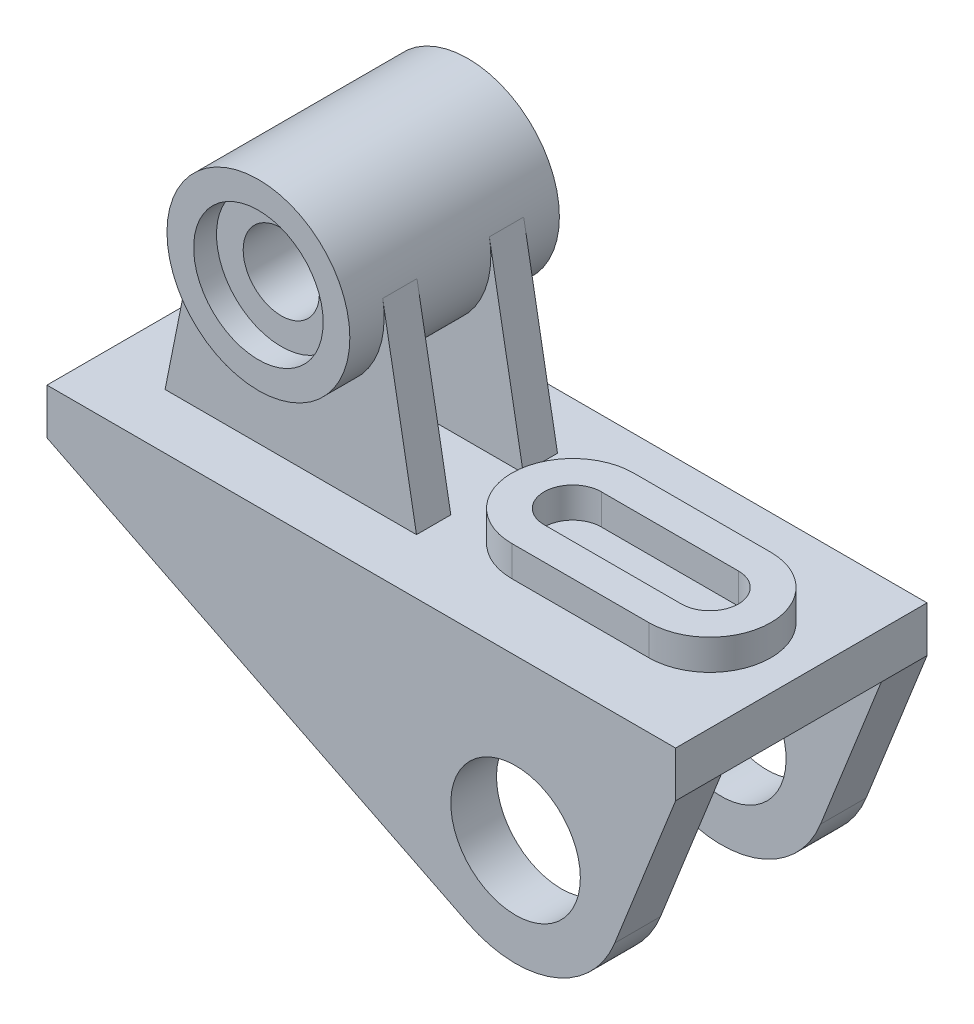
ISO-10303-21;
HEADER;
FILE_DESCRIPTION(('STEP AP214'),'2;1');
FILE_NAME('part.step','',(''),(''),'','','');
FILE_SCHEMA(('AUTOMOTIVE_DESIGN { 1 0 10303 214 1 1 1 1 }'));
ENDSEC;
DATA;
#1=APPLICATION_CONTEXT('core data for automotive mechanical design processes');
#2=APPLICATION_PROTOCOL_DEFINITION('international standard','automotive_design',2000,#1);
#3=PRODUCT_CONTEXT('',#1,'mechanical');
#4=PRODUCT('Part','Part','',(#3));
#5=PRODUCT_RELATED_PRODUCT_CATEGORY('part','',(#4));
#6=PRODUCT_DEFINITION_FORMATION('','',#4);
#7=PRODUCT_DEFINITION_CONTEXT('part definition',#1,'design');
#8=PRODUCT_DEFINITION('design','',#6,#7);
#9=PRODUCT_DEFINITION_SHAPE('','',#8);
#10=(LENGTH_UNIT() NAMED_UNIT(*) SI_UNIT(.MILLI.,.METRE.));
#11=(NAMED_UNIT(*) PLANE_ANGLE_UNIT() SI_UNIT($,.RADIAN.));
#12=(NAMED_UNIT(*) SI_UNIT($,.STERADIAN.) SOLID_ANGLE_UNIT());
#13=UNCERTAINTY_MEASURE_WITH_UNIT(LENGTH_MEASURE(1.E-05),#10,'distance_accuracy_value','');
#14=(GEOMETRIC_REPRESENTATION_CONTEXT(3) GLOBAL_UNCERTAINTY_ASSIGNED_CONTEXT((#13)) GLOBAL_UNIT_ASSIGNED_CONTEXT((#10,
#11,#12)) REPRESENTATION_CONTEXT('',''));
#15=CARTESIAN_POINT('',(0.,0.,0.));
#16=DIRECTION('',(0.,0.,1.));
#17=DIRECTION('',(1.,0.,0.));
#18=AXIS2_PLACEMENT_3D('',#15,#16,#17);
#19=CARTESIAN_POINT('',(50.,45.,27.5));
#20=DIRECTION('',(0.,0.,-1.));
#21=DIRECTION('',(-1.,0.,0.));
#22=AXIS2_PLACEMENT_3D('',#19,#20,#21);
#23=CYLINDRICAL_SURFACE('',#22,9.99999999999999);
#24=CARTESIAN_POINT('',(50.,45.,21.5));
#25=DIRECTION('',(0.,0.,1.));
#26=DIRECTION('',(1.,0.,0.));
#27=AXIS2_PLACEMENT_3D('',#24,#25,#26);
#28=CIRCLE('',#27,9.99999999999999);
#29=CARTESIAN_POINT('',(60.,45.,21.5));
#30=VERTEX_POINT('',#29);
#31=EDGE_CURVE('E248',#30,#30,#28,.T.);
#32=ORIENTED_EDGE('',*,*,#31,.T.);
#33=EDGE_LOOP('',(#32));
#34=FACE_BOUND('',#33,.T.);
#35=CARTESIAN_POINT('',(50.,45.,-21.5));
#36=DIRECTION('',(0.,0.,-1.));
#37=DIRECTION('',(-1.,0.,0.));
#38=AXIS2_PLACEMENT_3D('',#35,#36,#37);
#39=CIRCLE('',#38,9.99999999999999);
#40=CARTESIAN_POINT('',(40.,45.,-21.5));
#41=VERTEX_POINT('',#40);
#42=EDGE_CURVE('E43',#41,#41,#39,.T.);
#43=ORIENTED_EDGE('',*,*,#42,.T.);
#44=EDGE_LOOP('',(#43));
#45=FACE_BOUND('',#44,.T.);
#46=ADVANCED_FACE('F39',(#34,#45),#23,.F.);
#47=CARTESIAN_POINT('',(0.,0.,33.));
#48=DIRECTION('',(0.,-1.,0.));
#49=DIRECTION('',(0.,0.,-1.));
#50=AXIS2_PLACEMENT_3D('',#47,#48,#49);
#51=PLANE('',#50);
#52=DIRECTION('',(1.,0.,0.));
#53=VECTOR('',#52,1.);
#54=CARTESIAN_POINT('',(16.5,0.,9.5));
#55=LINE('',#54,#53);
#56=CARTESIAN_POINT('',(16.5,0.,9.5));
#57=VERTEX_POINT('',#56);
#58=CARTESIAN_POINT('',(82.5,0.,9.5));
#59=VERTEX_POINT('',#58);
#60=EDGE_CURVE('E268',#57,#59,#55,.T.);
#61=ORIENTED_EDGE('',*,*,#60,.T.);
#62=DIRECTION('',(0.,0.,1.));
#63=VECTOR('',#62,1.);
#64=CARTESIAN_POINT('',(82.5,0.,9.5));
#65=LINE('',#64,#63);
#66=CARTESIAN_POINT('',(82.5,0.,18.5));
#67=VERTEX_POINT('',#66);
#68=EDGE_CURVE('E289',#59,#67,#65,.T.);
#69=ORIENTED_EDGE('',*,*,#68,.T.);
#70=DIRECTION('',(1.,0.,0.));
#71=VECTOR('',#70,1.);
#72=CARTESIAN_POINT('',(16.5,0.,18.5));
#73=LINE('',#72,#71);
#74=CARTESIAN_POINT('',(16.5,0.,18.5));
#75=VERTEX_POINT('',#74);
#76=EDGE_CURVE('E276',#75,#67,#73,.T.);
#77=ORIENTED_EDGE('',*,*,#76,.F.);
#78=DIRECTION('',(0.,0.,1.));
#79=VECTOR('',#78,1.);
#80=CARTESIAN_POINT('',(16.5,0.,9.5));
#81=LINE('',#80,#79);
#82=EDGE_CURVE('E286',#57,#75,#81,.T.);
#83=ORIENTED_EDGE('',*,*,#82,.F.);
#84=EDGE_LOOP('',(#61,#69,#77,#83));
#85=FACE_BOUND('',#84,.T.);
#86=DIRECTION('',(-1.,0.,0.));
#87=VECTOR('',#86,1.);
#88=CARTESIAN_POINT('',(0.,0.,-33.));
#89=LINE('',#88,#87);
#90=CARTESIAN_POINT('',(165.,0.,-33.));
#91=VERTEX_POINT('',#90);
#92=CARTESIAN_POINT('',(0.,0.,-33.));
#93=VERTEX_POINT('',#92);
#94=EDGE_CURVE('E398',#91,#93,#89,.T.);
#95=ORIENTED_EDGE('',*,*,#94,.T.);
#96=DIRECTION('',(0.,0.,-1.));
#97=VECTOR('',#96,1.);
#98=CARTESIAN_POINT('',(0.,0.,33.));
#99=LINE('',#98,#97);
#100=CARTESIAN_POINT('',(0.,0.,33.));
#101=VERTEX_POINT('',#100);
#102=EDGE_CURVE('E408',#101,#93,#99,.T.);
#103=ORIENTED_EDGE('',*,*,#102,.F.);
#104=DIRECTION('',(-1.,0.,0.));
#105=VECTOR('',#104,1.);
#106=CARTESIAN_POINT('',(0.,0.,33.));
#107=LINE('',#106,#105);
#108=CARTESIAN_POINT('',(165.,0.,33.));
#109=VERTEX_POINT('',#108);
#110=EDGE_CURVE('E404',#109,#101,#107,.T.);
#111=ORIENTED_EDGE('',*,*,#110,.F.);
#112=DIRECTION('',(0.,0.,-1.));
#113=VECTOR('',#112,1.);
#114=CARTESIAN_POINT('',(165.,0.,33.));
#115=LINE('',#114,#113);
#116=EDGE_CURVE('E421',#109,#91,#115,.T.);
#117=ORIENTED_EDGE('',*,*,#116,.T.);
#118=EDGE_LOOP('',(#95,#103,#111,#117));
#119=FACE_BOUND('',#118,.T.);
#120=CARTESIAN_POINT('',(105.,0.,0.));
#121=DIRECTION('',(0.,1.,0.));
#122=DIRECTION('',(0.,0.,1.));
#123=AXIS2_PLACEMENT_3D('',#120,#121,#122);
#124=CIRCLE('',#123,16.);
#125=CARTESIAN_POINT('',(105.,0.,-16.));
#126=VERTEX_POINT('',#125);
#127=CARTESIAN_POINT('',(105.,0.,16.));
#128=VERTEX_POINT('',#127);
#129=EDGE_CURVE('E323',#126,#128,#124,.T.);
#130=ORIENTED_EDGE('',*,*,#129,.F.);
#131=DIRECTION('',(-1.,0.,0.));
#132=VECTOR('',#131,1.);
#133=CARTESIAN_POINT('',(105.,0.,-16.));
#134=LINE('',#133,#132);
#135=CARTESIAN_POINT('',(141.,0.,-16.));
#136=VERTEX_POINT('',#135);
#137=EDGE_CURVE('E327',#136,#126,#134,.T.);
#138=ORIENTED_EDGE('',*,*,#137,.F.);
#139=CARTESIAN_POINT('',(141.,0.,0.));
#140=DIRECTION('',(0.,1.,0.));
#141=DIRECTION('',(0.,0.,1.));
#142=AXIS2_PLACEMENT_3D('',#139,#140,#141);
#143=CIRCLE('',#142,16.);
#144=CARTESIAN_POINT('',(141.,0.,16.));
#145=VERTEX_POINT('',#144);
#146=EDGE_CURVE('E337',#145,#136,#143,.T.);
#147=ORIENTED_EDGE('',*,*,#146,.F.);
#148=DIRECTION('',(1.,0.,0.));
#149=VECTOR('',#148,1.);
#150=CARTESIAN_POINT('',(105.,0.,16.));
#151=LINE('',#150,#149);
#152=EDGE_CURVE('E340',#128,#145,#151,.T.);
#153=ORIENTED_EDGE('',*,*,#152,.F.);
#154=EDGE_LOOP('',(#130,#138,#147,#153));
#155=FACE_BOUND('',#154,.T.);
#156=DIRECTION('',(1.,0.,0.));
#157=VECTOR('',#156,1.);
#158=CARTESIAN_POINT('',(16.5,0.,-9.5));
#159=LINE('',#158,#157);
#160=CARTESIAN_POINT('',(16.5,0.,-9.5));
#161=VERTEX_POINT('',#160);
#162=CARTESIAN_POINT('',(82.5,0.,-9.5));
#163=VERTEX_POINT('',#162);
#164=EDGE_CURVE('E222',#161,#163,#159,.T.);
#165=ORIENTED_EDGE('',*,*,#164,.F.);
#166=DIRECTION('',(0.,0.,-1.));
#167=VECTOR('',#166,1.);
#168=CARTESIAN_POINT('',(16.5,0.,-9.5));
#169=LINE('',#168,#167);
#170=CARTESIAN_POINT('',(16.5,0.,-18.5));
#171=VERTEX_POINT('',#170);
#172=EDGE_CURVE('E252',#161,#171,#169,.T.);
#173=ORIENTED_EDGE('',*,*,#172,.T.);
#174=DIRECTION('',(1.,0.,0.));
#175=VECTOR('',#174,1.);
#176=CARTESIAN_POINT('',(16.5,0.,-18.5));
#177=LINE('',#176,#175);
#178=CARTESIAN_POINT('',(82.5,0.,-18.5));
#179=VERTEX_POINT('',#178);
#180=EDGE_CURVE('E237',#171,#179,#177,.T.);
#181=ORIENTED_EDGE('',*,*,#180,.T.);
#182=DIRECTION('',(0.,0.,-1.));
#183=VECTOR('',#182,1.);
#184=CARTESIAN_POINT('',(82.5,0.,-9.5));
#185=LINE('',#184,#183);
#186=EDGE_CURVE('E227',#163,#179,#185,.T.);
#187=ORIENTED_EDGE('',*,*,#186,.F.);
#188=EDGE_LOOP('',(#165,#173,#181,#187));
#189=FACE_BOUND('',#188,.T.);
#190=ADVANCED_FACE('F472',(#85,#119,#155,#189),#51,.F.);
#191=CARTESIAN_POINT('',(50.,45.,27.5));
#192=DIRECTION('',(0.,0.,-1.));
#193=DIRECTION('',(-1.,0.,0.));
#194=AXIS2_PLACEMENT_3D('',#191,#192,#193);
#195=CYLINDRICAL_SURFACE('',#194,24.);
#196=DIRECTION('',(0.,0.,1.));
#197=VECTOR('',#196,1.);
#198=CARTESIAN_POINT('',(73.6192033310231,49.25831351685,9.5));
#199=LINE('',#198,#197);
#200=CARTESIAN_POINT('',(73.6192033310231,49.25831351685,9.50000000000001));
#201=VERTEX_POINT('',#200);
#202=CARTESIAN_POINT('',(73.6192033310231,49.25831351685,18.5));
#203=VERTEX_POINT('',#202);
#204=EDGE_CURVE('E281',#201,#203,#199,.T.);
#205=ORIENTED_EDGE('',*,*,#204,.F.);
#206=CARTESIAN_POINT('',(50.,45.,9.5));
#207=DIRECTION('',(0.,0.,-1.));
#208=DIRECTION('',(1.,0.,0.));
#209=AXIS2_PLACEMENT_3D('',#206,#207,#208);
#210=CIRCLE('',#209,24.);
#211=CARTESIAN_POINT('',(26.4683154892939,49.7180318024145,9.50000000000001));
#212=VERTEX_POINT('',#211);
#213=EDGE_CURVE('E265',#201,#212,#210,.T.);
#214=ORIENTED_EDGE('',*,*,#213,.T.);
#215=DIRECTION('',(0.,0.,1.));
#216=VECTOR('',#215,1.);
#217=CARTESIAN_POINT('',(26.4683154892939,49.7180318024145,9.5));
#218=LINE('',#217,#216);
#219=CARTESIAN_POINT('',(26.4683154892939,49.7180318024145,18.5));
#220=VERTEX_POINT('',#219);
#221=EDGE_CURVE('E273',#212,#220,#218,.T.);
#222=ORIENTED_EDGE('',*,*,#221,.T.);
#223=CARTESIAN_POINT('',(50.,45.,18.5));
#224=DIRECTION('',(0.,0.,-1.));
#225=DIRECTION('',(1.,0.,0.));
#226=AXIS2_PLACEMENT_3D('',#223,#224,#225);
#227=CIRCLE('',#226,24.);
#228=EDGE_CURVE('E259',#203,#220,#227,.T.);
#229=ORIENTED_EDGE('',*,*,#228,.F.);
#230=EDGE_LOOP('',(#205,#214,#222,#229));
#231=FACE_BOUND('',#230,.T.);
#232=CARTESIAN_POINT('',(50.,45.,-27.5));
#233=DIRECTION('',(0.,0.,1.));
#234=DIRECTION('',(1.,0.,0.));
#235=AXIS2_PLACEMENT_3D('',#232,#233,#234);
#236=CIRCLE('',#235,24.);
#237=CARTESIAN_POINT('',(74.,45.,-27.5));
#238=VERTEX_POINT('',#237);
#239=EDGE_CURVE('E253',#238,#238,#236,.T.);
#240=ORIENTED_EDGE('',*,*,#239,.T.);
#241=EDGE_LOOP('',(#240));
#242=FACE_BOUND('',#241,.T.);
#243=CARTESIAN_POINT('',(50.,45.,27.5));
#244=DIRECTION('',(0.,0.,1.));
#245=DIRECTION('',(1.,0.,0.));
#246=AXIS2_PLACEMENT_3D('',#243,#244,#245);
#247=CIRCLE('',#246,24.);
#248=CARTESIAN_POINT('',(74.,45.,27.5));
#249=VERTEX_POINT('',#248);
#250=EDGE_CURVE('E258',#249,#249,#247,.T.);
#251=ORIENTED_EDGE('',*,*,#250,.F.);
#252=EDGE_LOOP('',(#251));
#253=FACE_BOUND('',#252,.T.);
#254=CARTESIAN_POINT('',(50.,45.,-9.5));
#255=DIRECTION('',(0.,0.,-1.));
#256=DIRECTION('',(1.,0.,0.));
#257=AXIS2_PLACEMENT_3D('',#254,#255,#256);
#258=CIRCLE('',#257,24.);
#259=CARTESIAN_POINT('',(73.6192033310231,49.25831351685,-9.5));
#260=VERTEX_POINT('',#259);
#261=CARTESIAN_POINT('',(26.4683154892939,49.7180318024145,-9.5));
#262=VERTEX_POINT('',#261);
#263=EDGE_CURVE('E218',#260,#262,#258,.T.);
#264=ORIENTED_EDGE('',*,*,#263,.F.);
#265=DIRECTION('',(0.,0.,-1.));
#266=VECTOR('',#265,1.);
#267=CARTESIAN_POINT('',(73.6192033310231,49.25831351685,-9.5));
#268=LINE('',#267,#266);
#269=CARTESIAN_POINT('',(73.6192033310231,49.25831351685,-18.5));
#270=VERTEX_POINT('',#269);
#271=EDGE_CURVE('E228',#260,#270,#268,.T.);
#272=ORIENTED_EDGE('',*,*,#271,.T.);
#273=CARTESIAN_POINT('',(50.,45.,-18.5));
#274=DIRECTION('',(0.,0.,-1.));
#275=DIRECTION('',(1.,0.,0.));
#276=AXIS2_PLACEMENT_3D('',#273,#274,#275);
#277=CIRCLE('',#276,24.);
#278=CARTESIAN_POINT('',(26.4683154892939,49.7180318024145,-18.5));
#279=VERTEX_POINT('',#278);
#280=EDGE_CURVE('E244',#270,#279,#277,.T.);
#281=ORIENTED_EDGE('',*,*,#280,.T.);
#282=DIRECTION('',(0.,0.,-1.));
#283=VECTOR('',#282,1.);
#284=CARTESIAN_POINT('',(26.4683154892939,49.7180318024145,-9.5));
#285=LINE('',#284,#283);
#286=EDGE_CURVE('E64',#262,#279,#285,.T.);
#287=ORIENTED_EDGE('',*,*,#286,.F.);
#288=EDGE_LOOP('',(#264,#272,#281,#287));
#289=FACE_BOUND('',#288,.T.);
#290=ADVANCED_FACE('F232',(#231,#242,#253,#289),#195,.T.);
#291=CARTESIAN_POINT('',(0.,-12.,33.));
#292=DIRECTION('',(0.445949175153248,0.895058284794983,0.));
#293=DIRECTION('',(-0.895058284794984,0.445949175153248,0.));
#294=AXIS2_PLACEMENT_3D('',#291,#292,#293);
#295=PLANE('',#294);
#296=DIRECTION('',(0.,0.,-1.));
#297=VECTOR('',#296,1.);
#298=CARTESIAN_POINT('',(0.,-12.,33.));
#299=LINE('',#298,#297);
#300=CARTESIAN_POINT('',(0.,-12.,33.));
#301=VERTEX_POINT('',#300);
#302=CARTESIAN_POINT('',(0.,-12.,21.));
#303=VERTEX_POINT('',#302);
#304=EDGE_CURVE('E11',#301,#303,#299,.T.);
#305=ORIENTED_EDGE('',*,*,#304,.T.);
#306=DIRECTION('',(0.895058284794984,-0.445949175153248,0.));
#307=VECTOR('',#306,1.);
#308=CARTESIAN_POINT('',(0.,-12.,21.));
#309=LINE('',#308,#307);
#310=CARTESIAN_POINT('',(110.513423095709,-67.0616319742595,21.));
#311=VERTEX_POINT('',#310);
#312=EDGE_CURVE('E385',#303,#311,#309,.T.);
#313=ORIENTED_EDGE('',*,*,#312,.T.);
#314=DIRECTION('',(0.,0.,-1.));
#315=VECTOR('',#314,1.);
#316=CARTESIAN_POINT('',(110.513423095709,-67.0616319742595,33.));
#317=LINE('',#316,#315);
#318=CARTESIAN_POINT('',(110.513423095709,-67.0616319742595,33.));
#319=VERTEX_POINT('',#318);
#320=EDGE_CURVE('E434',#319,#311,#317,.T.);
#321=ORIENTED_EDGE('',*,*,#320,.F.);
#322=DIRECTION('',(0.895058284794984,-0.445949175153248,0.));
#323=VECTOR('',#322,1.);
#324=CARTESIAN_POINT('',(0.,-12.,33.));
#325=LINE('',#324,#323);
#326=EDGE_CURVE('E392',#301,#319,#325,.T.);
#327=ORIENTED_EDGE('',*,*,#326,.F.);
#328=EDGE_LOOP('',(#305,#313,#321,#327));
#329=FACE_BOUND('',#328,.T.);
#330=ADVANCED_FACE('F497',(#329),#295,.F.);
#331=CARTESIAN_POINT('',(123.,-42.,33.));
#332=DIRECTION('',(0.,0.,-1.));
#333=DIRECTION('',(-1.,0.,0.));
#334=AXIS2_PLACEMENT_3D('',#331,#332,#333);
#335=CYLINDRICAL_SURFACE('',#334,28.);
#336=DIRECTION('',(0.,0.,-1.));
#337=VECTOR('',#336,1.);
#338=CARTESIAN_POINT('',(149.032106641509,-52.3116159647795,33.));
#339=LINE('',#338,#337);
#340=CARTESIAN_POINT('',(149.032106641509,-52.3116159647795,-21.));
#341=VERTEX_POINT('',#340);
#342=CARTESIAN_POINT('',(149.032106641509,-52.3116159647795,-33.));
#343=VERTEX_POINT('',#342);
#344=EDGE_CURVE('E429',#341,#343,#339,.T.);
#345=ORIENTED_EDGE('',*,*,#344,.F.);
#346=CARTESIAN_POINT('',(123.,-42.,-21.));
#347=DIRECTION('',(0.,0.,-1.));
#348=DIRECTION('',(0.,1.,0.));
#349=AXIS2_PLACEMENT_3D('',#346,#347,#348);
#350=CIRCLE('',#349,28.);
#351=CARTESIAN_POINT('',(110.513423095709,-67.0616319742595,-21.));
#352=VERTEX_POINT('',#351);
#353=EDGE_CURVE('E367',#341,#352,#350,.T.);
#354=ORIENTED_EDGE('',*,*,#353,.T.);
#355=CARTESIAN_POINT('',(110.513423095709,-67.0616319742595,-33.));
#356=VERTEX_POINT('',#355);
#357=EDGE_CURVE('E432',#352,#356,#317,.T.);
#358=ORIENTED_EDGE('',*,*,#357,.T.);
#359=CARTESIAN_POINT('',(123.,-42.,-33.));
#360=DIRECTION('',(0.,0.,1.));
#361=DIRECTION('',(1.,0.,0.));
#362=AXIS2_PLACEMENT_3D('',#359,#360,#361);
#363=CIRCLE('',#362,28.);
#364=EDGE_CURVE('E414',#356,#343,#363,.T.);
#365=ORIENTED_EDGE('',*,*,#364,.T.);
#366=EDGE_LOOP('',(#345,#354,#358,#365));
#367=FACE_BOUND('',#366,.T.);
#368=ADVANCED_FACE('F589',(#367),#335,.T.);
#369=CARTESIAN_POINT('',(165.,-12.,33.));
#370=DIRECTION('',(-0.929718094339613,0.368271998742124,0.));
#371=DIRECTION('',(-0.368271998742124,-0.929718094339613,0.));
#372=AXIS2_PLACEMENT_3D('',#369,#370,#371);
#373=PLANE('',#372);
#374=CARTESIAN_POINT('',(149.032106641509,-52.3116159647795,33.));
#375=VERTEX_POINT('',#374);
#376=CARTESIAN_POINT('',(149.032106641509,-52.3116159647795,21.));
#377=VERTEX_POINT('',#376);
#378=EDGE_CURVE('E431',#375,#377,#339,.T.);
#379=ORIENTED_EDGE('',*,*,#378,.T.);
#380=DIRECTION('',(0.368271998742124,0.929718094339613,0.));
#381=VECTOR('',#380,1.);
#382=CARTESIAN_POINT('',(165.,-12.,21.));
#383=LINE('',#382,#381);
#384=CARTESIAN_POINT('',(165.,-12.,21.));
#385=VERTEX_POINT('',#384);
#386=EDGE_CURVE('E380',#377,#385,#383,.T.);
#387=ORIENTED_EDGE('',*,*,#386,.T.);
#388=DIRECTION('',(0.,0.,-1.));
#389=VECTOR('',#388,1.);
#390=CARTESIAN_POINT('',(165.,-12.,33.));
#391=LINE('',#390,#389);
#392=CARTESIAN_POINT('',(165.,-12.,33.));
#393=VERTEX_POINT('',#392);
#394=EDGE_CURVE('E430',#393,#385,#391,.T.);
#395=ORIENTED_EDGE('',*,*,#394,.F.);
#396=DIRECTION('',(0.368271998742124,0.929718094339613,0.));
#397=VECTOR('',#396,1.);
#398=CARTESIAN_POINT('',(165.,-12.,33.));
#399=LINE('',#398,#397);
#400=EDGE_CURVE('E396',#375,#393,#399,.T.);
#401=ORIENTED_EDGE('',*,*,#400,.F.);
#402=EDGE_LOOP('',(#379,#387,#395,#401));
#403=FACE_BOUND('',#402,.T.);
#404=ADVANCED_FACE('F584',(#403),#373,.F.);
#405=CARTESIAN_POINT('',(123.,-42.,33.));
#406=DIRECTION('',(0.,0.,-1.));
#407=DIRECTION('',(-1.,0.,0.));
#408=AXIS2_PLACEMENT_3D('',#405,#406,#407);
#409=CYLINDRICAL_SURFACE('',#408,17.);
#410=CARTESIAN_POINT('',(123.,-42.,21.));
#411=DIRECTION('',(0.,0.,1.));
#412=DIRECTION('',(0.,-1.,0.));
#413=AXIS2_PLACEMENT_3D('',#410,#411,#412);
#414=CIRCLE('',#413,17.);
#415=CARTESIAN_POINT('',(123.,-59.,21.));
#416=VERTEX_POINT('',#415);
#417=EDGE_CURVE('E376',#416,#416,#414,.T.);
#418=ORIENTED_EDGE('',*,*,#417,.F.);
#419=EDGE_LOOP('',(#418));
#420=FACE_BOUND('',#419,.T.);
#421=CARTESIAN_POINT('',(123.,-42.,33.));
#422=DIRECTION('',(0.,0.,1.));
#423=DIRECTION('',(1.,0.,0.));
#424=AXIS2_PLACEMENT_3D('',#421,#422,#423);
#425=CIRCLE('',#424,17.);
#426=CARTESIAN_POINT('',(140.,-42.,33.));
#427=VERTEX_POINT('',#426);
#428=EDGE_CURVE('E387',#427,#427,#425,.T.);
#429=ORIENTED_EDGE('',*,*,#428,.T.);
#430=EDGE_LOOP('',(#429));
#431=FACE_BOUND('',#430,.T.);
#432=ADVANCED_FACE('F567',(#420,#431),#409,.F.);
#433=CARTESIAN_POINT('',(123.,-42.,33.));
#434=DIRECTION('',(0.,0.,1.));
#435=DIRECTION('',(1.,0.,0.));
#436=AXIS2_PLACEMENT_3D('',#433,#434,#435);
#437=PLANE('',#436);
#438=DIRECTION('',(0.,-1.,0.));
#439=VECTOR('',#438,1.);
#440=CARTESIAN_POINT('',(0.,0.,33.));
#441=LINE('',#440,#439);
#442=EDGE_CURVE('E395',#101,#301,#441,.T.);
#443=ORIENTED_EDGE('',*,*,#442,.T.);
#444=ORIENTED_EDGE('',*,*,#326,.T.);
#445=CARTESIAN_POINT('',(123.,-42.,33.));
#446=DIRECTION('',(0.,0.,1.));
#447=DIRECTION('',(1.,0.,0.));
#448=AXIS2_PLACEMENT_3D('',#445,#446,#447);
#449=CIRCLE('',#448,28.);
#450=EDGE_CURVE('E397',#319,#375,#449,.T.);
#451=ORIENTED_EDGE('',*,*,#450,.T.);
#452=ORIENTED_EDGE('',*,*,#400,.T.);
#453=DIRECTION('',(0.,1.,0.));
#454=VECTOR('',#453,1.);
#455=CARTESIAN_POINT('',(165.,0.,33.));
#456=LINE('',#455,#454);
#457=EDGE_CURVE('E405',#393,#109,#456,.T.);
#458=ORIENTED_EDGE('',*,*,#457,.T.);
#459=ORIENTED_EDGE('',*,*,#110,.T.);
#460=EDGE_LOOP('',(#443,#444,#451,#452,#458,#459));
#461=FACE_BOUND('',#460,.T.);
#462=ORIENTED_EDGE('',*,*,#428,.F.);
#463=EDGE_LOOP('',(#462));
#464=FACE_BOUND('',#463,.T.);
#465=ADVANCED_FACE('F570',(#461,#464),#437,.T.);
#466=CARTESIAN_POINT('',(123.,-42.,-33.));
#467=DIRECTION('',(0.,0.,1.));
#468=DIRECTION('',(1.,0.,0.));
#469=AXIS2_PLACEMENT_3D('',#466,#467,#468);
#470=PLANE('',#469);
#471=DIRECTION('',(0.,-1.,0.));
#472=VECTOR('',#471,1.);
#473=CARTESIAN_POINT('',(0.,0.,-33.));
#474=LINE('',#473,#472);
#475=CARTESIAN_POINT('',(0.,-12.,-33.));
#476=VERTEX_POINT('',#475);
#477=EDGE_CURVE('E386',#93,#476,#474,.T.);
#478=ORIENTED_EDGE('',*,*,#477,.F.);
#479=ORIENTED_EDGE('',*,*,#94,.F.);
#480=DIRECTION('',(0.,1.,0.));
#481=VECTOR('',#480,1.);
#482=CARTESIAN_POINT('',(165.,0.,-33.));
#483=LINE('',#482,#481);
#484=CARTESIAN_POINT('',(165.,-12.,-33.));
#485=VERTEX_POINT('',#484);
#486=EDGE_CURVE('E416',#485,#91,#483,.T.);
#487=ORIENTED_EDGE('',*,*,#486,.F.);
#488=DIRECTION('',(0.368271998742124,0.929718094339613,0.));
#489=VECTOR('',#488,1.);
#490=CARTESIAN_POINT('',(165.,-12.,-33.));
#491=LINE('',#490,#489);
#492=EDGE_CURVE('E411',#343,#485,#491,.T.);
#493=ORIENTED_EDGE('',*,*,#492,.F.);
#494=ORIENTED_EDGE('',*,*,#364,.F.);
#495=DIRECTION('',(0.895058284794984,-0.445949175153248,0.));
#496=VECTOR('',#495,1.);
#497=CARTESIAN_POINT('',(0.,-12.,-33.));
#498=LINE('',#497,#496);
#499=EDGE_CURVE('E409',#476,#356,#498,.T.);
#500=ORIENTED_EDGE('',*,*,#499,.F.);
#501=EDGE_LOOP('',(#478,#479,#487,#493,#494,#500));
#502=FACE_BOUND('',#501,.T.);
#503=CARTESIAN_POINT('',(123.,-42.,-33.));
#504=DIRECTION('',(0.,0.,1.));
#505=DIRECTION('',(1.,0.,0.));
#506=AXIS2_PLACEMENT_3D('',#503,#504,#505);
#507=CIRCLE('',#506,17.);
#508=CARTESIAN_POINT('',(140.,-42.,-33.));
#509=VERTEX_POINT('',#508);
#510=EDGE_CURVE('E384',#509,#509,#507,.T.);
#511=ORIENTED_EDGE('',*,*,#510,.T.);
#512=EDGE_LOOP('',(#511));
#513=FACE_BOUND('',#512,.T.);
#514=ADVANCED_FACE('F568',(#502,#513),#470,.F.);
#515=CARTESIAN_POINT('',(0.,0.,33.));
#516=DIRECTION('',(1.,0.,0.));
#517=DIRECTION('',(0.,0.,-1.));
#518=AXIS2_PLACEMENT_3D('',#515,#516,#517);
#519=PLANE('',#518);
#520=ORIENTED_EDGE('',*,*,#477,.T.);
#521=CARTESIAN_POINT('',(0.,-12.,-21.));
#522=VERTEX_POINT('',#521);
#523=EDGE_CURVE('E48',#522,#476,#299,.T.);
#524=ORIENTED_EDGE('',*,*,#523,.F.);
#525=DIRECTION('',(0.,0.,1.));
#526=VECTOR('',#525,1.);
#527=CARTESIAN_POINT('',(0.,-12.,21.));
#528=LINE('',#527,#526);
#529=EDGE_CURVE('E359',#522,#303,#528,.T.);
#530=ORIENTED_EDGE('',*,*,#529,.T.);
#531=ORIENTED_EDGE('',*,*,#304,.F.);
#532=ORIENTED_EDGE('',*,*,#442,.F.);
#533=ORIENTED_EDGE('',*,*,#102,.T.);
#534=EDGE_LOOP('',(#520,#524,#530,#531,#532,#533));
#535=FACE_BOUND('',#534,.T.);
#536=ADVANCED_FACE('F41',(#535),#519,.F.);
#537=ORIENTED_EDGE('',*,*,#357,.F.);
#538=DIRECTION('',(-0.895058284794984,0.445949175153248,0.));
#539=VECTOR('',#538,1.);
#540=CARTESIAN_POINT('',(0.,-12.,-21.));
#541=LINE('',#540,#539);
#542=EDGE_CURVE('E373',#352,#522,#541,.T.);
#543=ORIENTED_EDGE('',*,*,#542,.T.);
#544=ORIENTED_EDGE('',*,*,#523,.T.);
#545=ORIENTED_EDGE('',*,*,#499,.T.);
#546=EDGE_LOOP('',(#537,#543,#544,#545));
#547=FACE_BOUND('',#546,.T.);
#548=ADVANCED_FACE('F590',(#547),#295,.F.);
#549=CARTESIAN_POINT('',(123.,-42.,21.));
#550=DIRECTION('',(0.,0.,1.));
#551=DIRECTION('',(0.,-1.,0.));
#552=AXIS2_PLACEMENT_3D('',#549,#550,#551);
#553=CIRCLE('',#552,28.);
#554=EDGE_CURVE('E379',#311,#377,#553,.T.);
#555=ORIENTED_EDGE('',*,*,#554,.T.);
#556=ORIENTED_EDGE('',*,*,#378,.F.);
#557=ORIENTED_EDGE('',*,*,#450,.F.);
#558=ORIENTED_EDGE('',*,*,#320,.T.);
#559=EDGE_LOOP('',(#555,#556,#557,#558));
#560=FACE_BOUND('',#559,.T.);
#561=ADVANCED_FACE('F581',(#560),#335,.T.);
#562=CARTESIAN_POINT('',(165.,-12.,-21.));
#563=VERTEX_POINT('',#562);
#564=EDGE_CURVE('E426',#563,#485,#391,.T.);
#565=ORIENTED_EDGE('',*,*,#564,.F.);
#566=DIRECTION('',(-0.368271998742124,-0.929718094339613,0.));
#567=VECTOR('',#566,1.);
#568=CARTESIAN_POINT('',(165.,-12.,-21.));
#569=LINE('',#568,#567);
#570=EDGE_CURVE('E370',#563,#341,#569,.T.);
#571=ORIENTED_EDGE('',*,*,#570,.T.);
#572=ORIENTED_EDGE('',*,*,#344,.T.);
#573=ORIENTED_EDGE('',*,*,#492,.T.);
#574=EDGE_LOOP('',(#565,#571,#572,#573));
#575=FACE_BOUND('',#574,.T.);
#576=ADVANCED_FACE('F580',(#575),#373,.F.);
#577=CARTESIAN_POINT('',(165.,0.,33.));
#578=DIRECTION('',(-1.,0.,0.));
#579=DIRECTION('',(0.,0.,1.));
#580=AXIS2_PLACEMENT_3D('',#577,#578,#579);
#581=PLANE('',#580);
#582=ORIENTED_EDGE('',*,*,#486,.T.);
#583=ORIENTED_EDGE('',*,*,#116,.F.);
#584=ORIENTED_EDGE('',*,*,#457,.F.);
#585=ORIENTED_EDGE('',*,*,#394,.T.);
#586=DIRECTION('',(0.,0.,1.));
#587=VECTOR('',#586,1.);
#588=CARTESIAN_POINT('',(165.,-12.,21.));
#589=LINE('',#588,#587);
#590=EDGE_CURVE('E358',#563,#385,#589,.T.);
#591=ORIENTED_EDGE('',*,*,#590,.F.);
#592=ORIENTED_EDGE('',*,*,#564,.T.);
#593=EDGE_LOOP('',(#582,#583,#584,#585,#591,#592));
#594=FACE_BOUND('',#593,.T.);
#595=ADVANCED_FACE('F565',(#594),#581,.F.);
#596=CARTESIAN_POINT('',(123.,-42.,-21.));
#597=DIRECTION('',(0.,0.,-1.));
#598=DIRECTION('',(0.,1.,0.));
#599=AXIS2_PLACEMENT_3D('',#596,#597,#598);
#600=CIRCLE('',#599,17.);
#601=CARTESIAN_POINT('',(123.,-25.,-21.));
#602=VERTEX_POINT('',#601);
#603=EDGE_CURVE('E364',#602,#602,#600,.T.);
#604=ORIENTED_EDGE('',*,*,#603,.F.);
#605=EDGE_LOOP('',(#604));
#606=FACE_BOUND('',#605,.T.);
#607=ORIENTED_EDGE('',*,*,#510,.F.);
#608=EDGE_LOOP('',(#607));
#609=FACE_BOUND('',#608,.T.);
#610=ADVANCED_FACE('F557',(#606,#609),#409,.F.);
#611=CARTESIAN_POINT('',(0.,-12.,21.));
#612=DIRECTION('',(0.,0.,1.));
#613=DIRECTION('',(0.,-1.,0.));
#614=AXIS2_PLACEMENT_3D('',#611,#612,#613);
#615=PLANE('',#614);
#616=ORIENTED_EDGE('',*,*,#417,.T.);
#617=EDGE_LOOP('',(#616));
#618=FACE_BOUND('',#617,.T.);
#619=DIRECTION('',(1.,0.,0.));
#620=VECTOR('',#619,1.);
#621=CARTESIAN_POINT('',(0.,-12.,21.));
#622=LINE('',#621,#620);
#623=EDGE_CURVE('E361',#303,#385,#622,.T.);
#624=ORIENTED_EDGE('',*,*,#623,.T.);
#625=ORIENTED_EDGE('',*,*,#386,.F.);
#626=ORIENTED_EDGE('',*,*,#554,.F.);
#627=ORIENTED_EDGE('',*,*,#312,.F.);
#628=EDGE_LOOP('',(#624,#625,#626,#627));
#629=FACE_BOUND('',#628,.T.);
#630=ADVANCED_FACE('F558',(#618,#629),#615,.F.);
#631=CARTESIAN_POINT('',(0.,-12.,-21.));
#632=DIRECTION('',(0.,0.,-1.));
#633=DIRECTION('',(0.,1.,0.));
#634=AXIS2_PLACEMENT_3D('',#631,#632,#633);
#635=PLANE('',#634);
#636=ORIENTED_EDGE('',*,*,#603,.T.);
#637=EDGE_LOOP('',(#636));
#638=FACE_BOUND('',#637,.T.);
#639=ORIENTED_EDGE('',*,*,#353,.F.);
#640=ORIENTED_EDGE('',*,*,#570,.F.);
#641=DIRECTION('',(1.,0.,0.));
#642=VECTOR('',#641,1.);
#643=CARTESIAN_POINT('',(0.,-12.,-21.));
#644=LINE('',#643,#642);
#645=EDGE_CURVE('E356',#522,#563,#644,.T.);
#646=ORIENTED_EDGE('',*,*,#645,.F.);
#647=ORIENTED_EDGE('',*,*,#542,.F.);
#648=EDGE_LOOP('',(#639,#640,#646,#647));
#649=FACE_BOUND('',#648,.T.);
#650=ADVANCED_FACE('F555',(#638,#649),#635,.F.);
#651=CARTESIAN_POINT('',(0.,-12.,21.));
#652=DIRECTION('',(0.,1.,0.));
#653=DIRECTION('',(0.,0.,1.));
#654=AXIS2_PLACEMENT_3D('',#651,#652,#653);
#655=PLANE('',#654);
#656=ORIENTED_EDGE('',*,*,#590,.T.);
#657=ORIENTED_EDGE('',*,*,#623,.F.);
#658=ORIENTED_EDGE('',*,*,#529,.F.);
#659=ORIENTED_EDGE('',*,*,#645,.T.);
#660=EDGE_LOOP('',(#656,#657,#658,#659));
#661=FACE_BOUND('',#660,.T.);
#662=ADVANCED_FACE('F534',(#661),#655,.F.);
#663=CARTESIAN_POINT('',(105.,8.,0.));
#664=DIRECTION('',(0.,1.,0.));
#665=DIRECTION('',(0.,0.,1.));
#666=AXIS2_PLACEMENT_3D('',#663,#664,#665);
#667=PLANE('',#666);
#668=CARTESIAN_POINT('',(105.,8.,0.));
#669=DIRECTION('',(0.,1.,0.));
#670=DIRECTION('',(0.,0.,1.));
#671=AXIS2_PLACEMENT_3D('',#668,#669,#670);
#672=CIRCLE('',#671,16.);
#673=CARTESIAN_POINT('',(105.,8.,-16.));
#674=VERTEX_POINT('',#673);
#675=CARTESIAN_POINT('',(105.,8.,16.));
#676=VERTEX_POINT('',#675);
#677=EDGE_CURVE('E322',#674,#676,#672,.T.);
#678=ORIENTED_EDGE('',*,*,#677,.T.);
#679=DIRECTION('',(1.,0.,0.));
#680=VECTOR('',#679,1.);
#681=CARTESIAN_POINT('',(105.,8.,16.));
#682=LINE('',#681,#680);
#683=CARTESIAN_POINT('',(141.,8.,16.));
#684=VERTEX_POINT('',#683);
#685=EDGE_CURVE('E330',#676,#684,#682,.T.);
#686=ORIENTED_EDGE('',*,*,#685,.T.);
#687=CARTESIAN_POINT('',(141.,8.,0.));
#688=DIRECTION('',(0.,1.,0.));
#689=DIRECTION('',(0.,0.,1.));
#690=AXIS2_PLACEMENT_3D('',#687,#688,#689);
#691=CIRCLE('',#690,16.);
#692=CARTESIAN_POINT('',(141.,8.,-16.));
#693=VERTEX_POINT('',#692);
#694=EDGE_CURVE('E329',#684,#693,#691,.T.);
#695=ORIENTED_EDGE('',*,*,#694,.T.);
#696=DIRECTION('',(-1.,0.,0.));
#697=VECTOR('',#696,1.);
#698=CARTESIAN_POINT('',(105.,8.,-16.));
#699=LINE('',#698,#697);
#700=EDGE_CURVE('E335',#693,#674,#699,.T.);
#701=ORIENTED_EDGE('',*,*,#700,.T.);
#702=EDGE_LOOP('',(#678,#686,#695,#701));
#703=FACE_BOUND('',#702,.T.);
#704=DIRECTION('',(1.,0.,0.));
#705=VECTOR('',#704,1.);
#706=CARTESIAN_POINT('',(105.,8.,7.5));
#707=LINE('',#706,#705);
#708=CARTESIAN_POINT('',(105.,8.,7.5));
#709=VERTEX_POINT('',#708);
#710=CARTESIAN_POINT('',(141.,8.,7.49999999999999));
#711=VERTEX_POINT('',#710);
#712=EDGE_CURVE('E298',#709,#711,#707,.T.);
#713=ORIENTED_EDGE('',*,*,#712,.F.);
#714=CARTESIAN_POINT('',(105.,8.,0.));
#715=DIRECTION('',(0.,1.,0.));
#716=DIRECTION('',(0.,0.,1.));
#717=AXIS2_PLACEMENT_3D('',#714,#715,#716);
#718=CIRCLE('',#717,7.5);
#719=CARTESIAN_POINT('',(105.,8.,-7.5));
#720=VERTEX_POINT('',#719);
#721=EDGE_CURVE('E294',#720,#709,#718,.T.);
#722=ORIENTED_EDGE('',*,*,#721,.F.);
#723=DIRECTION('',(-1.,0.,0.));
#724=VECTOR('',#723,1.);
#725=CARTESIAN_POINT('',(105.,8.,-7.5));
#726=LINE('',#725,#724);
#727=CARTESIAN_POINT('',(141.,8.,-7.50000000000001));
#728=VERTEX_POINT('',#727);
#729=EDGE_CURVE('E304',#728,#720,#726,.T.);
#730=ORIENTED_EDGE('',*,*,#729,.F.);
#731=CARTESIAN_POINT('',(141.,8.,0.));
#732=DIRECTION('',(0.,1.,0.));
#733=DIRECTION('',(0.,0.,1.));
#734=AXIS2_PLACEMENT_3D('',#731,#732,#733);
#735=CIRCLE('',#734,7.5);
#736=EDGE_CURVE('E299',#711,#728,#735,.T.);
#737=ORIENTED_EDGE('',*,*,#736,.F.);
#738=EDGE_LOOP('',(#713,#722,#730,#737));
#739=FACE_BOUND('',#738,.T.);
#740=ADVANCED_FACE('F529',(#703,#739),#667,.T.);
#741=CARTESIAN_POINT('',(105.,8.,0.));
#742=DIRECTION('',(0.,-1.,0.));
#743=DIRECTION('',(0.,0.,-1.));
#744=AXIS2_PLACEMENT_3D('',#741,#742,#743);
#745=CYLINDRICAL_SURFACE('',#744,16.);
#746=ORIENTED_EDGE('',*,*,#129,.T.);
#747=DIRECTION('',(0.,-1.,0.));
#748=VECTOR('',#747,1.);
#749=CARTESIAN_POINT('',(105.,8.,16.));
#750=LINE('',#749,#748);
#751=EDGE_CURVE('E351',#676,#128,#750,.T.);
#752=ORIENTED_EDGE('',*,*,#751,.F.);
#753=ORIENTED_EDGE('',*,*,#677,.F.);
#754=DIRECTION('',(0.,-1.,0.));
#755=VECTOR('',#754,1.);
#756=CARTESIAN_POINT('',(105.,8.,-16.));
#757=LINE('',#756,#755);
#758=EDGE_CURVE('E331',#674,#126,#757,.T.);
#759=ORIENTED_EDGE('',*,*,#758,.T.);
#760=EDGE_LOOP('',(#746,#752,#753,#759));
#761=FACE_BOUND('',#760,.T.);
#762=ADVANCED_FACE('F531',(#761),#745,.T.);
#763=CARTESIAN_POINT('',(105.,8.,16.));
#764=DIRECTION('',(0.,0.,-1.));
#765=DIRECTION('',(-1.,0.,0.));
#766=AXIS2_PLACEMENT_3D('',#763,#764,#765);
#767=PLANE('',#766);
#768=ORIENTED_EDGE('',*,*,#152,.T.);
#769=DIRECTION('',(0.,-1.,0.));
#770=VECTOR('',#769,1.);
#771=CARTESIAN_POINT('',(141.,8.,16.));
#772=LINE('',#771,#770);
#773=EDGE_CURVE('E348',#684,#145,#772,.T.);
#774=ORIENTED_EDGE('',*,*,#773,.F.);
#775=ORIENTED_EDGE('',*,*,#685,.F.);
#776=ORIENTED_EDGE('',*,*,#751,.T.);
#777=EDGE_LOOP('',(#768,#774,#775,#776));
#778=FACE_BOUND('',#777,.T.);
#779=ADVANCED_FACE('F545',(#778),#767,.F.);
#780=CARTESIAN_POINT('',(141.,8.,0.));
#781=DIRECTION('',(0.,-1.,0.));
#782=DIRECTION('',(0.,0.,-1.));
#783=AXIS2_PLACEMENT_3D('',#780,#781,#782);
#784=CYLINDRICAL_SURFACE('',#783,16.);
#785=ORIENTED_EDGE('',*,*,#146,.T.);
#786=DIRECTION('',(0.,-1.,0.));
#787=VECTOR('',#786,1.);
#788=CARTESIAN_POINT('',(141.,8.,-16.));
#789=LINE('',#788,#787);
#790=EDGE_CURVE('E350',#693,#136,#789,.T.);
#791=ORIENTED_EDGE('',*,*,#790,.F.);
#792=ORIENTED_EDGE('',*,*,#694,.F.);
#793=ORIENTED_EDGE('',*,*,#773,.T.);
#794=EDGE_LOOP('',(#785,#791,#792,#793));
#795=FACE_BOUND('',#794,.T.);
#796=ADVANCED_FACE('F538',(#795),#784,.T.);
#797=CARTESIAN_POINT('',(105.,8.,-16.));
#798=DIRECTION('',(0.,0.,1.));
#799=DIRECTION('',(1.,0.,0.));
#800=AXIS2_PLACEMENT_3D('',#797,#798,#799);
#801=PLANE('',#800);
#802=ORIENTED_EDGE('',*,*,#137,.T.);
#803=ORIENTED_EDGE('',*,*,#758,.F.);
#804=ORIENTED_EDGE('',*,*,#700,.F.);
#805=ORIENTED_EDGE('',*,*,#790,.T.);
#806=EDGE_LOOP('',(#802,#803,#804,#805));
#807=FACE_BOUND('',#806,.T.);
#808=ADVANCED_FACE('F526',(#807),#801,.F.);
#809=CARTESIAN_POINT('',(105.,8.,0.));
#810=DIRECTION('',(0.,-1.,0.));
#811=DIRECTION('',(0.,0.,-1.));
#812=AXIS2_PLACEMENT_3D('',#809,#810,#811);
#813=CYLINDRICAL_SURFACE('',#812,7.5);
#814=CARTESIAN_POINT('',(105.,0.,0.));
#815=DIRECTION('',(0.,1.,0.));
#816=DIRECTION('',(0.,0.,1.));
#817=AXIS2_PLACEMENT_3D('',#814,#815,#816);
#818=CIRCLE('',#817,7.5);
#819=CARTESIAN_POINT('',(105.,0.,-7.5));
#820=VERTEX_POINT('',#819);
#821=CARTESIAN_POINT('',(105.,0.,7.5));
#822=VERTEX_POINT('',#821);
#823=EDGE_CURVE('E288',#820,#822,#818,.T.);
#824=ORIENTED_EDGE('',*,*,#823,.F.);
#825=DIRECTION('',(0.,-1.,0.));
#826=VECTOR('',#825,1.);
#827=CARTESIAN_POINT('',(105.,8.,-7.5));
#828=LINE('',#827,#826);
#829=EDGE_CURVE('E305',#720,#820,#828,.T.);
#830=ORIENTED_EDGE('',*,*,#829,.F.);
#831=ORIENTED_EDGE('',*,*,#721,.T.);
#832=DIRECTION('',(0.,-1.,0.));
#833=VECTOR('',#832,1.);
#834=CARTESIAN_POINT('',(105.,8.,7.5));
#835=LINE('',#834,#833);
#836=EDGE_CURVE('E319',#709,#822,#835,.T.);
#837=ORIENTED_EDGE('',*,*,#836,.T.);
#838=EDGE_LOOP('',(#824,#830,#831,#837));
#839=FACE_BOUND('',#838,.T.);
#840=ADVANCED_FACE('F525',(#839),#813,.F.);
#841=CARTESIAN_POINT('',(105.,8.,7.5));
#842=DIRECTION('',(0.,0.,-1.));
#843=DIRECTION('',(-1.,0.,0.));
#844=AXIS2_PLACEMENT_3D('',#841,#842,#843);
#845=PLANE('',#844);
#846=DIRECTION('',(1.,0.,0.));
#847=VECTOR('',#846,1.);
#848=CARTESIAN_POINT('',(105.,0.,7.5));
#849=LINE('',#848,#847);
#850=CARTESIAN_POINT('',(141.,0.,7.49999999999999));
#851=VERTEX_POINT('',#850);
#852=EDGE_CURVE('E307',#822,#851,#849,.T.);
#853=ORIENTED_EDGE('',*,*,#852,.F.);
#854=ORIENTED_EDGE('',*,*,#836,.F.);
#855=ORIENTED_EDGE('',*,*,#712,.T.);
#856=DIRECTION('',(0.,-1.,0.));
#857=VECTOR('',#856,1.);
#858=CARTESIAN_POINT('',(141.,8.,7.49999999999999));
#859=LINE('',#858,#857);
#860=EDGE_CURVE('E318',#711,#851,#859,.T.);
#861=ORIENTED_EDGE('',*,*,#860,.T.);
#862=EDGE_LOOP('',(#853,#854,#855,#861));
#863=FACE_BOUND('',#862,.T.);
#864=ADVANCED_FACE('F517',(#863),#845,.T.);
#865=CARTESIAN_POINT('',(141.,8.,0.));
#866=DIRECTION('',(0.,-1.,0.));
#867=DIRECTION('',(0.,0.,-1.));
#868=AXIS2_PLACEMENT_3D('',#865,#866,#867);
#869=CYLINDRICAL_SURFACE('',#868,7.5);
#870=CARTESIAN_POINT('',(141.,0.,0.));
#871=DIRECTION('',(0.,1.,0.));
#872=DIRECTION('',(0.,0.,1.));
#873=AXIS2_PLACEMENT_3D('',#870,#871,#872);
#874=CIRCLE('',#873,7.5);
#875=CARTESIAN_POINT('',(141.,0.,-7.50000000000001));
#876=VERTEX_POINT('',#875);
#877=EDGE_CURVE('E309',#851,#876,#874,.T.);
#878=ORIENTED_EDGE('',*,*,#877,.F.);
#879=ORIENTED_EDGE('',*,*,#860,.F.);
#880=ORIENTED_EDGE('',*,*,#736,.T.);
#881=DIRECTION('',(0.,-1.,0.));
#882=VECTOR('',#881,1.);
#883=CARTESIAN_POINT('',(141.,8.,-7.50000000000001));
#884=LINE('',#883,#882);
#885=EDGE_CURVE('E316',#728,#876,#884,.T.);
#886=ORIENTED_EDGE('',*,*,#885,.T.);
#887=EDGE_LOOP('',(#878,#879,#880,#886));
#888=FACE_BOUND('',#887,.T.);
#889=ADVANCED_FACE('F518',(#888),#869,.F.);
#890=CARTESIAN_POINT('',(105.,8.,-7.5));
#891=DIRECTION('',(0.,0.,1.));
#892=DIRECTION('',(1.,0.,0.));
#893=AXIS2_PLACEMENT_3D('',#890,#891,#892);
#894=PLANE('',#893);
#895=DIRECTION('',(-1.,0.,0.));
#896=VECTOR('',#895,1.);
#897=CARTESIAN_POINT('',(105.,0.,-7.5));
#898=LINE('',#897,#896);
#899=EDGE_CURVE('E300',#876,#820,#898,.T.);
#900=ORIENTED_EDGE('',*,*,#899,.F.);
#901=ORIENTED_EDGE('',*,*,#885,.F.);
#902=ORIENTED_EDGE('',*,*,#729,.T.);
#903=ORIENTED_EDGE('',*,*,#829,.T.);
#904=EDGE_LOOP('',(#900,#901,#902,#903));
#905=FACE_BOUND('',#904,.T.);
#906=ADVANCED_FACE('F511',(#905),#894,.T.);
#907=ORIENTED_EDGE('',*,*,#899,.T.);
#908=ORIENTED_EDGE('',*,*,#823,.T.);
#909=ORIENTED_EDGE('',*,*,#852,.T.);
#910=ORIENTED_EDGE('',*,*,#877,.T.);
#911=EDGE_LOOP('',(#907,#908,#909,#910));
#912=FACE_BOUND('',#911,.T.);
#913=ADVANCED_FACE('F481',(#912),#51,.F.);
#914=CARTESIAN_POINT('',(73.6192033310231,49.25831351685,9.5));
#915=DIRECTION('',(0.984133472125962,0.17742972986875,0.));
#916=DIRECTION('',(-0.17742972986875,0.984133472125962,0.));
#917=AXIS2_PLACEMENT_3D('',#914,#915,#916);
#918=PLANE('',#917);
#919=DIRECTION('',(-0.17742972986875,0.984133472125962,0.));
#920=VECTOR('',#919,1.);
#921=CARTESIAN_POINT('',(73.6192033310231,49.25831351685,18.5));
#922=LINE('',#921,#920);
#923=EDGE_CURVE('E264',#67,#203,#922,.T.);
#924=ORIENTED_EDGE('',*,*,#923,.F.);
#925=ORIENTED_EDGE('',*,*,#68,.F.);
#926=DIRECTION('',(-0.17742972986875,0.984133472125962,0.));
#927=VECTOR('',#926,1.);
#928=CARTESIAN_POINT('',(73.6192033310231,49.25831351685,9.5));
#929=LINE('',#928,#927);
#930=EDGE_CURVE('E271',#59,#201,#929,.T.);
#931=ORIENTED_EDGE('',*,*,#930,.T.);
#932=ORIENTED_EDGE('',*,*,#204,.T.);
#933=EDGE_LOOP('',(#924,#925,#931,#932));
#934=FACE_BOUND('',#933,.T.);
#935=ADVANCED_FACE('F508',(#934),#918,.T.);
#936=CARTESIAN_POINT('',(26.4683154892939,49.7180318024145,9.5));
#937=DIRECTION('',(-0.980486854612754,0.196584658433939,0.));
#938=DIRECTION('',(-0.196584658433939,-0.980486854612754,0.));
#939=AXIS2_PLACEMENT_3D('',#936,#937,#938);
#940=PLANE('',#939);
#941=DIRECTION('',(-0.196584658433939,-0.980486854612754,0.));
#942=VECTOR('',#941,1.);
#943=CARTESIAN_POINT('',(26.4683154892939,49.7180318024145,18.5));
#944=LINE('',#943,#942);
#945=EDGE_CURVE('E280',#220,#75,#944,.T.);
#946=ORIENTED_EDGE('',*,*,#945,.F.);
#947=ORIENTED_EDGE('',*,*,#221,.F.);
#948=DIRECTION('',(-0.196584658433939,-0.980486854612754,0.));
#949=VECTOR('',#948,1.);
#950=CARTESIAN_POINT('',(26.4683154892939,49.7180318024145,9.5));
#951=LINE('',#950,#949);
#952=EDGE_CURVE('E262',#212,#57,#951,.T.);
#953=ORIENTED_EDGE('',*,*,#952,.T.);
#954=ORIENTED_EDGE('',*,*,#82,.T.);
#955=EDGE_LOOP('',(#946,#947,#953,#954));
#956=FACE_BOUND('',#955,.T.);
#957=ADVANCED_FACE('F503',(#956),#940,.T.);
#958=CARTESIAN_POINT('',(50.,45.,9.5));
#959=DIRECTION('',(0.,0.,1.));
#960=DIRECTION('',(1.,0.,0.));
#961=AXIS2_PLACEMENT_3D('',#958,#959,#960);
#962=PLANE('',#961);
#963=ORIENTED_EDGE('',*,*,#213,.F.);
#964=ORIENTED_EDGE('',*,*,#930,.F.);
#965=ORIENTED_EDGE('',*,*,#60,.F.);
#966=ORIENTED_EDGE('',*,*,#952,.F.);
#967=EDGE_LOOP('',(#963,#964,#965,#966));
#968=FACE_BOUND('',#967,.T.);
#969=ADVANCED_FACE('F499',(#968),#962,.F.);
#970=CARTESIAN_POINT('',(50.,45.,18.5));
#971=DIRECTION('',(0.,0.,1.));
#972=DIRECTION('',(1.,0.,0.));
#973=AXIS2_PLACEMENT_3D('',#970,#971,#972);
#974=PLANE('',#973);
#975=ORIENTED_EDGE('',*,*,#228,.T.);
#976=ORIENTED_EDGE('',*,*,#945,.T.);
#977=ORIENTED_EDGE('',*,*,#76,.T.);
#978=ORIENTED_EDGE('',*,*,#923,.T.);
#979=EDGE_LOOP('',(#975,#976,#977,#978));
#980=FACE_BOUND('',#979,.T.);
#981=ADVANCED_FACE('F487',(#980),#974,.T.);
#982=CARTESIAN_POINT('',(50.,45.,27.5));
#983=DIRECTION('',(0.,0.,1.));
#984=DIRECTION('',(1.,0.,0.));
#985=AXIS2_PLACEMENT_3D('',#982,#983,#984);
#986=PLANE('',#985);
#987=CARTESIAN_POINT('',(50.,45.,27.5));
#988=DIRECTION('',(0.,0.,1.));
#989=DIRECTION('',(1.,0.,0.));
#990=AXIS2_PLACEMENT_3D('',#987,#988,#989);
#991=CIRCLE('',#990,17.);
#992=CARTESIAN_POINT('',(67.,45.,27.5));
#993=VERTEX_POINT('',#992);
#994=EDGE_CURVE('E239',#993,#993,#991,.T.);
#995=ORIENTED_EDGE('',*,*,#994,.F.);
#996=EDGE_LOOP('',(#995));
#997=FACE_BOUND('',#996,.T.);
#998=ORIENTED_EDGE('',*,*,#250,.T.);
#999=EDGE_LOOP('',(#998));
#1000=FACE_BOUND('',#999,.T.);
#1001=ADVANCED_FACE('F484',(#997,#1000),#986,.T.);
#1002=CARTESIAN_POINT('',(50.,45.,-27.5));
#1003=DIRECTION('',(0.,0.,1.));
#1004=DIRECTION('',(1.,0.,0.));
#1005=AXIS2_PLACEMENT_3D('',#1002,#1003,#1004);
#1006=PLANE('',#1005);
#1007=CARTESIAN_POINT('',(50.,45.,-27.5));
#1008=DIRECTION('',(0.,0.,1.));
#1009=DIRECTION('',(1.,0.,0.));
#1010=AXIS2_PLACEMENT_3D('',#1007,#1008,#1009);
#1011=CIRCLE('',#1010,17.);
#1012=CARTESIAN_POINT('',(67.,45.,-27.5));
#1013=VERTEX_POINT('',#1012);
#1014=EDGE_CURVE('E447',#1013,#1013,#1011,.T.);
#1015=ORIENTED_EDGE('',*,*,#1014,.T.);
#1016=EDGE_LOOP('',(#1015));
#1017=FACE_BOUND('',#1016,.T.);
#1018=ORIENTED_EDGE('',*,*,#239,.F.);
#1019=EDGE_LOOP('',(#1018));
#1020=FACE_BOUND('',#1019,.T.);
#1021=ADVANCED_FACE('F488',(#1017,#1020),#1006,.F.);
#1022=CARTESIAN_POINT('',(26.4683154892939,49.7180318024145,-9.5));
#1023=DIRECTION('',(0.980486854612754,-0.196584658433939,0.));
#1024=DIRECTION('',(0.196584658433939,0.980486854612754,0.));
#1025=AXIS2_PLACEMENT_3D('',#1022,#1023,#1024);
#1026=PLANE('',#1025);
#1027=DIRECTION('',(-0.196584658433939,-0.980486854612754,0.));
#1028=VECTOR('',#1027,1.);
#1029=CARTESIAN_POINT('',(26.4683154892939,49.7180318024145,-18.5));
#1030=LINE('',#1029,#1028);
#1031=EDGE_CURVE('E235',#279,#171,#1030,.T.);
#1032=ORIENTED_EDGE('',*,*,#1031,.T.);
#1033=ORIENTED_EDGE('',*,*,#172,.F.);
#1034=DIRECTION('',(-0.196584658433939,-0.980486854612754,0.));
#1035=VECTOR('',#1034,1.);
#1036=CARTESIAN_POINT('',(26.4683154892939,49.7180318024145,-9.5));
#1037=LINE('',#1036,#1035);
#1038=EDGE_CURVE('E233',#262,#161,#1037,.T.);
#1039=ORIENTED_EDGE('',*,*,#1038,.F.);
#1040=ORIENTED_EDGE('',*,*,#286,.T.);
#1041=EDGE_LOOP('',(#1032,#1033,#1039,#1040));
#1042=FACE_BOUND('',#1041,.T.);
#1043=ADVANCED_FACE('F495',(#1042),#1026,.F.);
#1044=CARTESIAN_POINT('',(73.6192033310231,49.25831351685,-9.5));
#1045=DIRECTION('',(-0.984133472125962,-0.17742972986875,0.));
#1046=DIRECTION('',(0.17742972986875,-0.984133472125962,0.));
#1047=AXIS2_PLACEMENT_3D('',#1044,#1045,#1046);
#1048=PLANE('',#1047);
#1049=DIRECTION('',(-0.17742972986875,0.984133472125962,0.));
#1050=VECTOR('',#1049,1.);
#1051=CARTESIAN_POINT('',(73.6192033310231,49.25831351685,-18.5));
#1052=LINE('',#1051,#1050);
#1053=EDGE_CURVE('E57',#179,#270,#1052,.T.);
#1054=ORIENTED_EDGE('',*,*,#1053,.T.);
#1055=ORIENTED_EDGE('',*,*,#271,.F.);
#1056=DIRECTION('',(-0.17742972986875,0.984133472125962,0.));
#1057=VECTOR('',#1056,1.);
#1058=CARTESIAN_POINT('',(73.6192033310231,49.25831351685,-9.5));
#1059=LINE('',#1058,#1057);
#1060=EDGE_CURVE('E214',#163,#260,#1059,.T.);
#1061=ORIENTED_EDGE('',*,*,#1060,.F.);
#1062=ORIENTED_EDGE('',*,*,#186,.T.);
#1063=EDGE_LOOP('',(#1054,#1055,#1061,#1062));
#1064=FACE_BOUND('',#1063,.T.);
#1065=ADVANCED_FACE('F230',(#1064),#1048,.F.);
#1066=CARTESIAN_POINT('',(50.,45.,-9.5));
#1067=DIRECTION('',(0.,0.,-1.));
#1068=DIRECTION('',(1.,0.,0.));
#1069=AXIS2_PLACEMENT_3D('',#1066,#1067,#1068);
#1070=PLANE('',#1069);
#1071=ORIENTED_EDGE('',*,*,#263,.T.);
#1072=ORIENTED_EDGE('',*,*,#1038,.T.);
#1073=ORIENTED_EDGE('',*,*,#164,.T.);
#1074=ORIENTED_EDGE('',*,*,#1060,.T.);
#1075=EDGE_LOOP('',(#1071,#1072,#1073,#1074));
#1076=FACE_BOUND('',#1075,.T.);
#1077=ADVANCED_FACE('F220',(#1076),#1070,.F.);
#1078=CARTESIAN_POINT('',(50.,45.,-18.5));
#1079=DIRECTION('',(0.,0.,-1.));
#1080=DIRECTION('',(1.,0.,0.));
#1081=AXIS2_PLACEMENT_3D('',#1078,#1079,#1080);
#1082=PLANE('',#1081);
#1083=ORIENTED_EDGE('',*,*,#280,.F.);
#1084=ORIENTED_EDGE('',*,*,#1053,.F.);
#1085=ORIENTED_EDGE('',*,*,#180,.F.);
#1086=ORIENTED_EDGE('',*,*,#1031,.F.);
#1087=EDGE_LOOP('',(#1083,#1084,#1085,#1086));
#1088=FACE_BOUND('',#1087,.T.);
#1089=ADVANCED_FACE('F640',(#1088),#1082,.T.);
#1090=CARTESIAN_POINT('',(50.,45.,21.5));
#1091=DIRECTION('',(0.,0.,1.));
#1092=DIRECTION('',(1.,0.,0.));
#1093=AXIS2_PLACEMENT_3D('',#1090,#1091,#1092);
#1094=CYLINDRICAL_SURFACE('',#1093,17.);
#1095=CARTESIAN_POINT('',(50.,45.,21.5));
#1096=DIRECTION('',(0.,0.,1.));
#1097=DIRECTION('',(1.,0.,0.));
#1098=AXIS2_PLACEMENT_3D('',#1095,#1096,#1097);
#1099=CIRCLE('',#1098,17.);
#1100=CARTESIAN_POINT('',(67.,45.,21.5));
#1101=VERTEX_POINT('',#1100);
#1102=EDGE_CURVE('E445',#1101,#1101,#1099,.T.);
#1103=ORIENTED_EDGE('',*,*,#1102,.F.);
#1104=EDGE_LOOP('',(#1103));
#1105=FACE_BOUND('',#1104,.T.);
#1106=ORIENTED_EDGE('',*,*,#994,.T.);
#1107=EDGE_LOOP('',(#1106));
#1108=FACE_BOUND('',#1107,.T.);
#1109=ADVANCED_FACE('F650',(#1105,#1108),#1094,.F.);
#1110=CARTESIAN_POINT('',(50.,45.,21.5));
#1111=DIRECTION('',(0.,0.,1.));
#1112=DIRECTION('',(1.,0.,0.));
#1113=AXIS2_PLACEMENT_3D('',#1110,#1111,#1112);
#1114=PLANE('',#1113);
#1115=ORIENTED_EDGE('',*,*,#31,.F.);
#1116=EDGE_LOOP('',(#1115));
#1117=FACE_BOUND('',#1116,.T.);
#1118=ORIENTED_EDGE('',*,*,#1102,.T.);
#1119=EDGE_LOOP('',(#1118));
#1120=FACE_BOUND('',#1119,.T.);
#1121=ADVANCED_FACE('F470',(#1117,#1120),#1114,.T.);
#1122=CARTESIAN_POINT('',(50.,45.,-21.5));
#1123=DIRECTION('',(0.,0.,-1.));
#1124=DIRECTION('',(-1.,0.,0.));
#1125=AXIS2_PLACEMENT_3D('',#1122,#1123,#1124);
#1126=CYLINDRICAL_SURFACE('',#1125,17.);
#1127=CARTESIAN_POINT('',(50.,45.,-21.5));
#1128=DIRECTION('',(0.,0.,1.));
#1129=DIRECTION('',(1.,0.,0.));
#1130=AXIS2_PLACEMENT_3D('',#1127,#1128,#1129);
#1131=CIRCLE('',#1130,17.);
#1132=CARTESIAN_POINT('',(67.,45.,-21.5));
#1133=VERTEX_POINT('',#1132);
#1134=EDGE_CURVE('E452',#1133,#1133,#1131,.T.);
#1135=ORIENTED_EDGE('',*,*,#1134,.T.);
#1136=EDGE_LOOP('',(#1135));
#1137=FACE_BOUND('',#1136,.T.);
#1138=ORIENTED_EDGE('',*,*,#1014,.F.);
#1139=EDGE_LOOP('',(#1138));
#1140=FACE_BOUND('',#1139,.T.);
#1141=ADVANCED_FACE('F464',(#1137,#1140),#1126,.F.);
#1142=CARTESIAN_POINT('',(50.,45.,-21.5));
#1143=DIRECTION('',(0.,0.,-1.));
#1144=DIRECTION('',(1.,0.,0.));
#1145=AXIS2_PLACEMENT_3D('',#1142,#1143,#1144);
#1146=PLANE('',#1145);
#1147=ORIENTED_EDGE('',*,*,#42,.F.);
#1148=EDGE_LOOP('',(#1147));
#1149=FACE_BOUND('',#1148,.T.);
#1150=ORIENTED_EDGE('',*,*,#1134,.F.);
#1151=EDGE_LOOP('',(#1150));
#1152=FACE_BOUND('',#1151,.T.);
#1153=ADVANCED_FACE('F463',(#1149,#1152),#1146,.T.);
#1154=CLOSED_SHELL('',(#46,#190,#290,#330,#368,#404,#432,#465,#514,#536,#548,#561,#576,#595,
#610,#630,#650,#662,#740,#762,#779,#796,#808,#840,#864,#889,#906,#913,#935,#957,#969,#981,#1001,
#1021,#1043,#1065,#1077,#1089,#1109,#1121,#1141,#1153));
#1155=MANIFOLD_SOLID_BREP('B2',#1154);
#1156=ADVANCED_BREP_SHAPE_REPRESENTATION('',(#18,#1155),#14);
#1157=SHAPE_DEFINITION_REPRESENTATION(#9,#1156);
ENDSEC;
END-ISO-10303-21;
